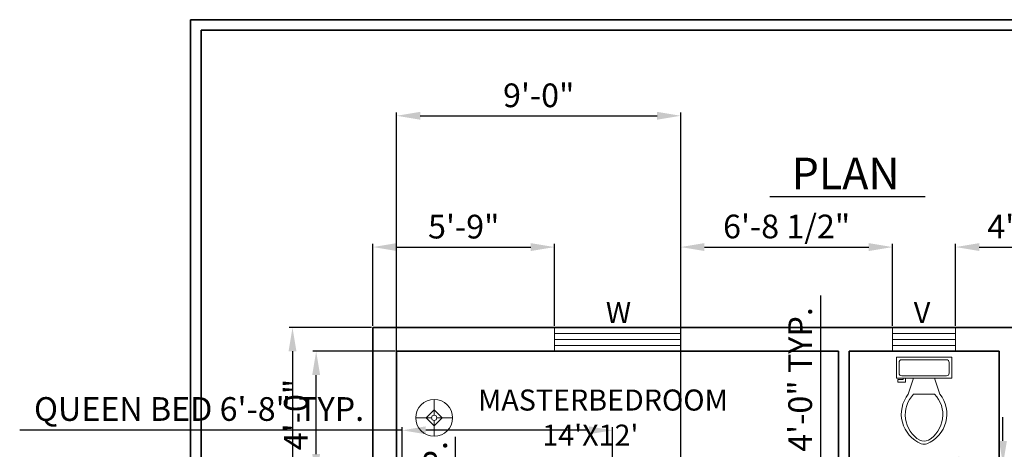
# Model space of a CAD drawing. Units: inches. Extents: x 2396 to 4051, y 1419 to 2191.
# Tile 4 of 7: x 2396 to 2770, y 2028 to 2191. Entities that reach past the tile are written whole.
import ezdxf

# ---------------------------------------------------------------- set-up
doc = ezdxf.new("R2010")
doc.units = ezdxf.units.IN
doc.layers.add('A-ANNO-TEXT', color=114, linetype='Continuous', lineweight=18, true_color=0x139b48)
doc.layers.add('A-GLAZ', color=52, linetype='Continuous', lineweight=18, true_color=0xc8c92d)
for name, color, linetype, lineweight in [('A-ANNO-TITL', 7, 'Continuous', 25), ('A-ANNO-TTLB', 7, 'Continuous', 35), ('A-AREA-IDEN', 6, 'Continuous', 18), ('A-FLOR-FIXT', 9, 'Continuous', 18), ('A-FURN', 8, 'Continuous', 18), ('A-WALL', 7, 'Continuous', 35), ('S-ANNO-DIMS', 2, 'Continuous', 18)]:
    doc.layers.add(name, color=color, linetype=linetype, lineweight=lineweight)
doc.styles.get("Standard").update_dxf_attribs({"font": 'arial.ttf'})
doc.dimstyles.new('ISO-25', dxfattribs={"dimtxt": 9, "dimasz": 9, "dimexe": 1.25, "dimexo": 0.625, "dimgap": 2, "dimtad": 1, "dimdec": 1, "dimlunit": 4, "dimtxsty": 'Standard', "dimcen": 2.5, "dimadec": 0, "dimazin": 0, "dimtfac": 1, "dimtdec": 1, "dimtmove": 0, "dimatfit": 3, "dimfxl": 1, "dimarcsym": 0})

# ---------------------------------------------------------------- blocks, each defined once
blk = doc.blocks.new('Lamp - Table')
for p, q in [((0, 7), (0, 1)), ((-1, 0), (-7, 0)), ((0, 3), (-3, 0)), ((-3, 0), (0, -3)), ((3, 0), (0, 3)), ((0, -3), (3, 0)), ((1, 0), (7, 0)), ((0, -1), (0, -7))]:
    blk.add_line(p, q)
for radius in [7, 1]:
    blk.add_circle((0, 0), radius)
blk = doc.blocks.new('Toilet - top')
for p, q in [((9.5, -6), (9.5, -2)), ((-10, -8.5), (-8, -8.5)), ((-10, -9.5), (-10, -8.5)), ((-7, -9.5), (-10, -9.5)), ((-8, -8.5), (-8, -8)), ((-7, -8), (-7, -9.5)), ((-4, -8), (-6, -14)), ((4, -8), (6, -14)), ((4, -14), (-4, -14))]:
    blk.add_line(p, q)
blk.add_lwpolyline([(10.5, -8), (10.5, 0), (-10.5, 0), (-10.5, -8)], close=True)
for points in [[(-9.5, -2), (-9.5, -6)], [(8.5, -1), (-8.5, -1)], [(-8.5, -7), (8.5, -7)]]:
    blk.add_lwpolyline(points)
for centre, radius, start, end in [((-8.62, -1.88), 0.884, 81.8699, 188.1301), ((8.62, -1.88), 0.884, 351.8699, 98.1301), ((-8.62, -6.12), 0.884, 171.8699, 278.1301), ((8.62, -6.12), 0.884, 261.8699, 8.1301), ((3.52, -21.58), 12.17, 141.4691, 247.9714), ((4.2, -21.82), 11.33, 136.3677, 238.9468), ((-3.52, -21.58), 12.17, 292.0284, 38.5307), ((-4.2, -21.82), 11.33, 301.053, 43.6321), ((0, -27.88), 4, 245.7318, 294.2682), ((0, -29), 4, 254.8605, 285.1395)]:
    blk.add_arc(centre, radius, start, end)
blk = doc.blocks.new('WIN-W-48IN')
for p, q in [((0, 0), (0, 9)), ((48, 0), (48, 9)), ((0, 6.75), (48, 6.75)), ((0, 4.5), (48, 4.5)), ((0, 2.25), (48, 2.25))]:
    blk.add_line(p, q)
blk = doc.blocks.new('VENT-V-24IN')
for p, q in [((0, 0), (0, 9)), ((24, 0), (24, 9)), ((0, 6.75), (24, 6.75)), ((0, 4.5), (24, 4.5)), ((0, 2.25), (24, 2.25))]:
    blk.add_line(p, q)
blk = doc.blocks.new('*D41')
at = {"layer": 'Defpoints', "color": 0, "transparency": 16777216}
for p in [(2559.21, 1956.76), (2561.31, 1956.76), (2559.21, 1942.76)]:
    blk.add_point(p, dxfattribs=at)
at = {"layer": 'S-ANNO-DIMS', "color": 0, "lineweight": -2, "transparency": 16777216}
for p, q in [((2561.31, 1965.76), (2561.31, 2032.77)), ((2559.83, 1956.76), (2562.56, 1956.76)), ((2561.31, 1942.76), (2561.31, 1956.76)), ((2559.83, 1942.76), (2562.56, 1942.76)), ((2561.31, 1933.76), (2561.31, 1924.76))]:
    blk.add_line(p, q, dxfattribs=at)
at = {"layer": 'S-ANNO-DIMS', "color": 0, "transparency": 16777216}
for points in [[(2559.81, 1965.76), (2562.81, 1965.76), (2561.31, 1956.76)], [(2559.81, 1933.76), (2562.81, 1933.76), (2561.31, 1942.76)]]:
    blk.add_solid(points, dxfattribs=at)
at = {"layer": 'S-ANNO-DIMS', "color": 0, "transparency": 16777216, "insert": (2554.79, 2003.76), "char_height": 9, "attachment_point": 5, "rotation": 90}
blk.add_mtext('1\'-2" TYP.', dxfattribs=at)
blk = doc.blocks.new('*D46')
at = {"layer": 'Defpoints', "color": 0, "transparency": 16777216}
for p in [(2541.07, 2035.3), (2541.07, 2023.3), (2621.07, 2023.3)]:
    blk.add_point(p, dxfattribs=at)
at = {"layer": 'S-ANNO-DIMS', "color": 0, "lineweight": -2, "transparency": 16777216}
for p, q in [((2541.07, 2023.93), (2541.07, 2036.55)), ((2621.07, 2023.93), (2621.07, 2036.55)), ((2541.07, 2035.3), (2395.68, 2035.3)), ((2612.07, 2035.3), (2550.07, 2035.3))]:
    blk.add_line(p, q, dxfattribs=at)
at = {"layer": 'S-ANNO-DIMS', "color": 0, "transparency": 16777216}
for points in [[(2550.07, 2036.8), (2550.07, 2033.8), (2541.07, 2035.3)], [(2612.07, 2036.8), (2612.07, 2033.8), (2621.07, 2035.3)]]:
    blk.add_solid(points, dxfattribs=at)
at = {"layer": 'S-ANNO-DIMS', "color": 0, "transparency": 16777216, "insert": (2463.87, 2042.23), "char_height": 9, "attachment_point": 5}
blk.add_mtext('QUEEN BED 6\'-8" TYP.', dxfattribs=at)
blk = doc.blocks.new('*D50')
at = {"layer": 'Defpoints', "color": 0, "transparency": 16777216}
for p in [(2767.98, 2022.3), (2767.98, 2012.3), (2769.48, 2012.3)]:
    blk.add_point(p, dxfattribs=at)
at = {"layer": 'S-ANNO-DIMS', "color": 0, "lineweight": -2, "transparency": 16777216}
for p, q in [((2769.48, 2031.3), (2769.48, 2040.3)), ((2768.61, 2022.3), (2770.73, 2022.3)), ((2769.48, 2022.3), (2769.48, 2012.3)), ((2768.61, 2012.3), (2770.73, 2012.3)), ((2769.48, 2003.3), (2769.48, 1859.68))]:
    blk.add_line(p, q, dxfattribs=at)
at = {"layer": 'S-ANNO-DIMS', "color": 0, "transparency": 16777216}
for points in [[(2767.98, 2031.3), (2770.98, 2031.3), (2769.48, 2022.3)], [(2767.98, 2003.3), (2770.98, 2003.3), (2769.48, 2012.3)]]:
    blk.add_solid(points, dxfattribs=at)
at = {"layer": 'S-ANNO-DIMS', "color": 0, "transparency": 16777216, "insert": (2762.83, 1926.99), "char_height": 9, "attachment_point": 5, "rotation": 90}
blk.add_mtext('BASIN TAP 0\'-10" TYP.', dxfattribs=at)
blk = doc.blocks.new('*D51')
at = {"layer": 'Defpoints', "color": 0, "transparency": 16777216}
for p in [(2761.48, 2022.3), (2767.98, 2023.8), (2767.98, 2022.3)]:
    blk.add_point(p, dxfattribs=at)
at = {"layer": 'S-ANNO-DIMS', "color": 0, "lineweight": -2, "transparency": 16777216}
for p, q in [((2761.48, 2022.93), (2761.48, 2025.05)), ((2767.98, 2022.93), (2767.98, 2025.05)), ((2752.48, 2023.8), (2743.48, 2023.8)), ((2761.48, 2023.8), (2767.98, 2023.8)), ((2776.98, 2023.8), (2865.81, 2023.8))]:
    blk.add_line(p, q, dxfattribs=at)
at = {"layer": 'S-ANNO-DIMS', "color": 0, "transparency": 16777216}
for points in [[(2752.48, 2025.3), (2752.48, 2022.3), (2761.48, 2023.8)], [(2776.98, 2025.3), (2776.98, 2022.3), (2767.98, 2023.8)]]:
    blk.add_solid(points, dxfattribs=at)
at = {"layer": 'S-ANNO-DIMS', "color": 0, "transparency": 16777216, "insert": (2825.9, 2030.45), "char_height": 9, "attachment_point": 5}
blk.add_mtext('0\'-6 1/2" TYP.', dxfattribs=at)
blk = doc.blocks.new('*D56')
at = {"layer": 'Defpoints', "color": 0, "transparency": 16777216}
for p in [(2692.98, 1965.3), (2700.18, 1965.3), (2692.98, 1917.3)]:
    blk.add_point(p, dxfattribs=at)
at = {"layer": 'S-ANNO-DIMS', "color": 0, "lineweight": -2, "transparency": 16777216}
for p, q in [((2700.18, 1965.3), (2700.18, 2086.5)), ((2693.61, 1965.3), (2701.43, 1965.3)), ((2700.18, 1926.3), (2700.18, 1956.3)), ((2693.61, 1917.3), (2701.43, 1917.3))]:
    blk.add_line(p, q, dxfattribs=at)
at = {"layer": 'S-ANNO-DIMS', "color": 0, "transparency": 16777216}
for points in [[(2698.68, 1956.3), (2701.68, 1956.3), (2700.18, 1965.3)], [(2698.68, 1926.3), (2701.68, 1926.3), (2700.18, 1917.3)]]:
    blk.add_solid(points, dxfattribs=at)
at = {"layer": 'S-ANNO-DIMS', "color": 0, "transparency": 16777216, "insert": (2693.53, 2030.4), "char_height": 9, "attachment_point": 5, "rotation": 90}
blk.add_mtext('DOOR D 4\'-0" TYP.', dxfattribs=at)
blk = doc.blocks.new('*D77')
at = {"layer": 'Defpoints', "color": 0, "transparency": 16777216}
for p in [(2529.98, 2074.3), (2499.38, 1534.3), (2774.98, 1534.3)]:
    blk.add_point(p, dxfattribs=at)
at = {"layer": 'S-ANNO-DIMS', "color": 0, "lineweight": -2, "transparency": 16777216}
for p, q in [((2529.36, 2074.3), (2498.13, 2074.3)), ((2499.38, 2065.3), (2499.38, 1543.3)), ((2774.36, 1534.3), (2498.13, 1534.3))]:
    blk.add_line(p, q, dxfattribs=at)
at = {"layer": 'S-ANNO-DIMS', "color": 0, "transparency": 16777216}
for points in [[(2497.88, 2065.3), (2500.88, 2065.3), (2499.38, 2074.3)], [(2497.88, 1543.3), (2500.88, 1543.3), (2499.38, 1534.3)]]:
    blk.add_solid(points, dxfattribs=at)
at = {"layer": 'S-ANNO-DIMS', "color": 0, "transparency": 16777216, "insert": (2492.79, 1804.3), "char_height": 9, "attachment_point": 5, "rotation": 90}
blk.add_mtext('45\'-0"', dxfattribs=at)
blk = doc.blocks.new('*D85')
at = {"layer": 'Defpoints', "color": 0, "transparency": 16777216}
for p in [(2598.98, 2104.9), (2529.98, 2074.3), (2598.98, 2074.3)]:
    blk.add_point(p, dxfattribs=at)
at = {"layer": 'S-ANNO-DIMS', "color": 0, "lineweight": -2, "transparency": 16777216}
for p, q in [((2529.98, 2074.93), (2529.98, 2106.15)), ((2538.98, 2104.9), (2589.98, 2104.9)), ((2598.98, 2074.93), (2598.98, 2106.15))]:
    blk.add_line(p, q, dxfattribs=at)
at = {"layer": 'S-ANNO-DIMS', "color": 0, "transparency": 16777216}
for points in [[(2538.98, 2106.4), (2538.98, 2103.4), (2529.98, 2104.9)], [(2589.98, 2106.4), (2589.98, 2103.4), (2598.98, 2104.9)]]:
    blk.add_solid(points, dxfattribs=at)
at = {"layer": 'S-ANNO-DIMS', "color": 0, "transparency": 16777216, "insert": (2564.48, 2111.5), "char_height": 9, "attachment_point": 5}
blk.add_mtext('5\'-9"', dxfattribs=at)
blk = doc.blocks.new('*D86')
at = {"layer": 'Defpoints', "color": 0, "transparency": 16777216}
for p in [(2727.48, 2104.9), (2646.98, 2074.3), (2727.48, 2074.3)]:
    blk.add_point(p, dxfattribs=at)
at = {"layer": 'S-ANNO-DIMS', "color": 0, "lineweight": -2, "transparency": 16777216}
for p, q in [((2646.98, 2074.93), (2646.98, 2106.15)), ((2655.98, 2104.9), (2718.48, 2104.9)), ((2727.48, 2074.93), (2727.48, 2106.15))]:
    blk.add_line(p, q, dxfattribs=at)
at = {"layer": 'S-ANNO-DIMS', "color": 0, "transparency": 16777216}
for points in [[(2655.98, 2106.4), (2655.98, 2103.4), (2646.98, 2104.9)], [(2718.48, 2106.4), (2718.48, 2103.4), (2727.48, 2104.9)]]:
    blk.add_solid(points, dxfattribs=at)
at = {"layer": 'S-ANNO-DIMS', "color": 0, "transparency": 16777216, "insert": (2687.23, 2111.55), "char_height": 9, "attachment_point": 5}
blk.add_mtext('6\'-8 1/2"', dxfattribs=at)
blk = doc.blocks.new('*D87')
at = {"layer": 'Defpoints', "color": 0, "transparency": 16777216}
for p in [(2809.48, 2104.9), (2751.48, 2074.3), (2809.48, 2074.3)]:
    blk.add_point(p, dxfattribs=at)
at = {"layer": 'S-ANNO-DIMS', "color": 0, "lineweight": -2, "transparency": 16777216}
for p, q in [((2751.48, 2074.93), (2751.48, 2106.15)), ((2760.48, 2104.9), (2800.48, 2104.9)), ((2809.48, 2074.93), (2809.48, 2106.15))]:
    blk.add_line(p, q, dxfattribs=at)
at = {"layer": 'S-ANNO-DIMS', "color": 0, "transparency": 16777216}
for points in [[(2760.48, 2106.4), (2760.48, 2103.4), (2751.48, 2104.9)], [(2800.48, 2106.4), (2800.48, 2103.4), (2809.48, 2104.9)]]:
    blk.add_solid(points, dxfattribs=at)
at = {"layer": 'S-ANNO-DIMS', "color": 0, "transparency": 16777216, "insert": (2780.48, 2111.5), "char_height": 9, "attachment_point": 5}
blk.add_mtext('4\'-10"', dxfattribs=at)
blk = doc.blocks.new('*D91')
at = {"layer": 'Defpoints', "color": 0, "transparency": 16777216}
for p in [(2508.38, 2065.3), (2538.98, 2065.3), (2538.98, 2017.3)]:
    blk.add_point(p, dxfattribs=at)
at = {"layer": 'S-ANNO-DIMS', "color": 0, "lineweight": -2, "transparency": 16777216}
for p, q in [((2538.36, 2065.3), (2507.13, 2065.3)), ((2508.38, 2026.3), (2508.38, 2056.3)), ((2538.36, 2017.3), (2507.13, 2017.3))]:
    blk.add_line(p, q, dxfattribs=at)
at = {"layer": 'S-ANNO-DIMS', "color": 0, "transparency": 16777216}
for points in [[(2506.88, 2056.3), (2509.88, 2056.3), (2508.38, 2065.3)], [(2506.88, 2026.3), (2509.88, 2026.3), (2508.38, 2017.3)]]:
    blk.add_solid(points, dxfattribs=at)
at = {"layer": 'S-ANNO-DIMS', "color": 0, "transparency": 16777216, "insert": (2501.79, 2041.3), "char_height": 9, "attachment_point": 5, "rotation": 90}
blk.add_mtext('4\'-0"', dxfattribs=at)
blk = doc.blocks.new('*D95')
at = {"layer": 'Defpoints', "color": 0, "transparency": 16777216}
for p in [(2646.98, 2154.77), (2538.98, 1853.3), (2646.98, 1853.3)]:
    blk.add_point(p, dxfattribs=at)
at = {"layer": 'S-ANNO-DIMS', "color": 0, "lineweight": -2, "transparency": 16777216}
for p, q in [((2538.98, 1853.93), (2538.98, 2156.02)), ((2646.98, 1853.93), (2646.98, 2156.02)), ((2547.98, 2154.77), (2637.98, 2154.77))]:
    blk.add_line(p, q, dxfattribs=at)
at = {"layer": 'S-ANNO-DIMS', "color": 0, "transparency": 16777216}
for points in [[(2547.98, 2156.27), (2547.98, 2153.27), (2538.98, 2154.77)], [(2637.98, 2156.27), (2637.98, 2153.27), (2646.98, 2154.77)]]:
    blk.add_solid(points, dxfattribs=at)
at = {"layer": 'S-ANNO-DIMS', "color": 0, "transparency": 16777216, "insert": (2592.98, 2161.37), "char_height": 9, "attachment_point": 5}
blk.add_mtext('9\'-0"', dxfattribs=at)

msp = doc.modelspace()

# ---------------------------------------------------------------- linework, layer by layer
at = {"layer": 'A-ANNO-TITL'}
msp.add_line((2680.79, 2124.17), (2739.87, 2124.17), dxfattribs=at)
at = {"layer": 'A-ANNO-TTLB'}
for points in [[(2460.66, 2191.26), (4051.21, 2191.26), (4051.21, 1469.82), (2460.66, 1469.82)], [(2464.66, 2187.26), (4047.21, 2187.26), (4047.21, 1473.82), (2464.66, 1473.82)]]:
    msp.add_lwpolyline(points, close=True, dxfattribs=at)
at = {"layer": 'A-WALL'}
for p, q in [((2529.98, 1632.3), (2529.98, 2074.3)), ((2529.98, 2074.3), (2903.98, 2074.3)), ((2538.98, 2065.3), (2706.98, 2065.3)), ((2538.98, 1921.3), (2538.98, 2065.3)), ((2706.98, 2065.3), (2706.98, 1921.3)), ((2710.98, 2065.3), (2710.98, 1969.3)), ((2710.98, 2065.3), (2767.98, 2065.3)), ((2767.98, 2065.3), (2767.98, 1969.3))]:
    msp.add_line(p, q, dxfattribs=at)

# ---------------------------------------------------------------- block references
at = {"layer": 'A-FLOR-FIXT'}
msp.add_blockref('Toilet - top', (2739.48, 2063.05), dxfattribs=at)
at = {"layer": 'A-FURN'}
msp.add_blockref('Lamp - Table', (2553.25, 2040.04), dxfattribs=at)
at = {"layer": 'A-GLAZ'}
for name, p in [('WIN-W-48IN', (2598.98, 2065.3)), ('VENT-V-24IN', (2727.48, 2065.3))]:
    msp.add_blockref(name, p, dxfattribs=at)

# ---------------------------------------------------------------- texts
at = {"layer": 'A-ANNO-TEXT', "char_height": 8, "attachment_point": 1}
for s, insert in [('W', (2618.51, 2084.02)), ('V', (2735.57, 2084.01))]:
    msp.add_mtext_dynamic_manual_height_columns(s, width=139.3028, gutter_width=12.5, heights=[0], dxfattribs=dict(at, insert=insert))
at = {"layer": 'A-ANNO-TITL', "insert": (2689.12, 2138.87), "char_height": 12, "attachment_point": 1}
msp.add_mtext_dynamic_manual_height_columns('{\\fArial|b1|i0|c0|p34;PLAN}', width=349.2365, gutter_width=12.5, heights=[0], dxfattribs=at)
at = {"layer": 'A-AREA-IDEN', "insert": (2569.91, 2050.8), "char_height": 8, "attachment_point": 1}
msp.add_mtext_dynamic_manual_height_columns("MASTERBEDROOM\\P          14'X12'", width=139.3028, gutter_width=12.5, heights=[0], dxfattribs=at)

# ---------------------------------------------------------------- dimensions: what is measured, and where the dimension line sits
at = {"layer": 'S-ANNO-DIMS'}
for base, p1, p2, picture, middle in [((2646.98, 2154.77), (2538.98, 1853.3), (2646.98, 1853.3), '*D95', (2592.98, 2161.37)), ((2598.98, 2104.9), (2529.98, 2074.3), (2598.98, 2074.3), '*D85', (2564.48, 2111.5)), ((2809.48, 2104.9), (2751.48, 2074.3), (2809.48, 2074.3), '*D87', (2780.48, 2111.5))]:
    dim = msp.add_linear_dim(base=base, p1=p1, p2=p2, dimstyle='ISO-25', override={"dimdec": 1, "dimlfac": 1, "dimrnd": 0, "dimzin": 1, "dimdsep": 46, "dimlunit": 4, "dimfrac": 2}, dxfattribs=at)
    dim.commit()
    dim.dimension.update_dxf_attribs({"geometry": picture, "text_midpoint": middle})
for base, p1, p2, angle, picture, middle in [((2727.48, 2104.9), (2646.98, 2074.3), (2727.48, 2074.3), 0, '*D86', (2687.23, 2111.55)), ((2499.38, 1534.3), (2529.98, 2074.3), (2774.98, 1534.3), 90, '*D77', (2492.79, 1804.3)), ((2508.38, 2065.3), (2538.98, 2017.3), (2538.98, 2065.3), 90, '*D91', (2501.79, 2041.3))]:
    dim = msp.add_linear_dim(base=base, p1=p1, p2=p2, angle=angle, dimstyle='ISO-25', override={"dimdec": 1, "dimlfac": 1, "dimrnd": 0, "dimzin": 1, "dimdsep": 46, "dimlunit": 4, "dimfrac": 2}, dxfattribs=at)
    dim.commit()
    dim.dimension.update_dxf_attribs({"geometry": picture, "text_midpoint": middle})
for base, p1, p2, angle, text, picture, middle in [((2700.18, 1965.3), (2692.98, 1917.3), (2692.98, 1965.3), 90, 'DOOR D <> TYP.', '*D56', (2693.53, 2030.4)), ((2541.07, 2035.3), (2621.07, 2023.3), (2541.07, 2023.3), 180, 'QUEEN BED <> TYP.', '*D46', (2463.87, 2042.23)), ((2769.48, 2012.3), (2767.98, 2022.3), (2767.98, 2012.3), 270, 'BASIN TAP <> TYP.', '*D50', (2762.83, 1926.99)), ((2561.31, 1956.76), (2559.21, 1942.76), (2559.21, 1956.76), 90, '<> TYP.', '*D41', (2554.79, 2003.76))]:
    dim = msp.add_linear_dim(base=base, p1=p1, p2=p2, angle=angle, text=text, dimstyle='ISO-25', override={"dimdec": 1, "dimlfac": 1, "dimrnd": 0, "dimzin": 1, "dimdsep": 46, "dimlunit": 4, "dimfrac": 2}, dxfattribs=at)
    dim.commit()
    dim.dimension.update_dxf_attribs({"geometry": picture, "text_midpoint": middle})
dim = msp.add_linear_dim(base=(2767.98, 2023.8), p1=(2761.48, 2022.3), p2=(2767.98, 2022.3), text='<> TYP.', dimstyle='ISO-25', override={"dimdec": 1, "dimlfac": 1, "dimrnd": 0, "dimzin": 1, "dimdsep": 46, "dimlunit": 4, "dimfrac": 2}, dxfattribs=at)
dim.commit()
dim.dimension.update_dxf_attribs({"geometry": '*D51', "text_midpoint": (2825.9, 2030.45)})

doc.saveas('drawing.dxf')
